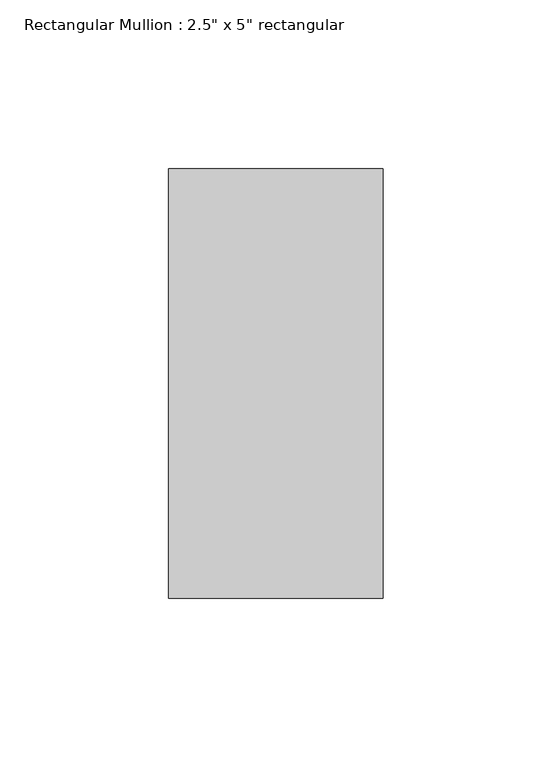
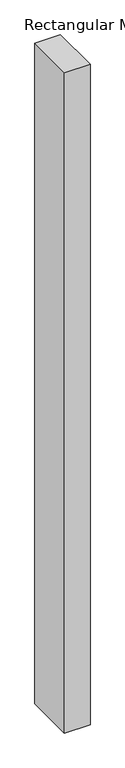
"""IFC4 building model written with IfcOpenShell, lengths in millimetres: member geometry."""

from ifc_helpers import new_model, si_unit, frame, origin, place, context, project, spatial, polyline, outline, extrude, source, transform, mapped, element, save


def member_b289f3f9(model_context):
    return source(origin(), model_context, "Body", "SweptSolid", [
        extrude(outline(polyline([(0.0, 63.5), (0.0, -63.5), (-63.5, -63.5), (-63.5, 63.5), (0.0, 63.5)])), frame((0.0, 0.0, -1732.6965064), z_axis=(0.0, 0.0, 1.0), x_axis=(1.0, 0.0, 0.0)), (0.0, 0.0, 1.0), 1732.6965064),
    ])


if __name__ == "__main__":
    model = new_model("IFC4")
    model_context = context("Model", 3, world=origin())
    ifc_project = project(units=[si_unit("LENGTHUNIT", "METRE", prefix="MILLI")], contexts=[model_context])
    site = spatial("IfcSite", under=ifc_project)
    building = spatial("IfcBuilding", under=site)
    placement = place(None, origin())
    member_shape = member_b289f3f9(model_context)
    element("IfcMember", 1, ObjectType="Rectangular Mullion : 2.5\" x 5\" rectangular", at=placement, inside=building, context=model_context, shape_type="MappedRepresentation", body=[
        mapped(member_shape, transform((0.0, 0.0, 0.0), x_axis=(1.0, 0.0, 0.0), y_axis=(0.0, 1.0, 0.0), z_axis=(0.0, 0.0, 1.0))),
    ])
    save(model, "model.ifc")

# Revit data of these elements
# Type "Rectangular Mullion : 2.5\" x 5\" rectangular"
#   built-in parameter 1007304 = 0.416667 (stored number, unit not read)
#   built-in parameter 1007301 = 0.104167 (stored number, unit not read)
#   built-in parameter 1007300 = 0.104167 (stored number, unit not read)
# Element 1 (IfcMember, "Rectangular Mullion : 2.5\" x 5\" rectangular")
#   Materials on its faces: "Aluminum"
# Materials
#   "Aluminum": class "Metal", colour RGB 247 247 247, transparency 0, Description = "Aluminum 6061", Cost = 0
